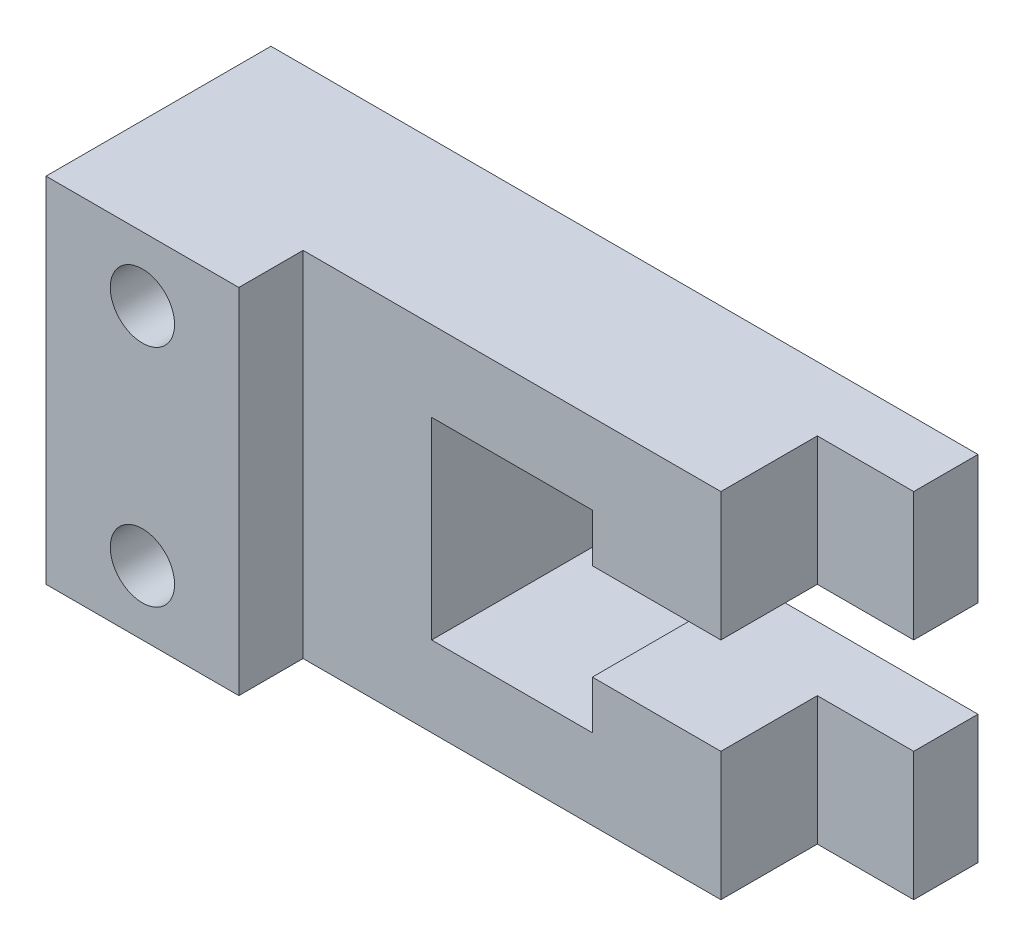
ISO-10303-21;
HEADER;
FILE_DESCRIPTION(('STEP AP214'),'2;1');
FILE_NAME('part.step','',(''),(''),'','','');
FILE_SCHEMA(('AUTOMOTIVE_DESIGN { 1 0 10303 214 1 1 1 1 }'));
ENDSEC;
DATA;
#1=APPLICATION_CONTEXT('core data for automotive mechanical design processes');
#2=APPLICATION_PROTOCOL_DEFINITION('international standard','automotive_design',2000,#1);
#3=PRODUCT_CONTEXT('',#1,'mechanical');
#4=PRODUCT('Part','Part','',(#3));
#5=PRODUCT_RELATED_PRODUCT_CATEGORY('part','',(#4));
#6=PRODUCT_DEFINITION_FORMATION('','',#4);
#7=PRODUCT_DEFINITION_CONTEXT('part definition',#1,'design');
#8=PRODUCT_DEFINITION('design','',#6,#7);
#9=PRODUCT_DEFINITION_SHAPE('','',#8);
#10=(LENGTH_UNIT() NAMED_UNIT(*) SI_UNIT(.MILLI.,.METRE.));
#11=(NAMED_UNIT(*) PLANE_ANGLE_UNIT() SI_UNIT($,.RADIAN.));
#12=(NAMED_UNIT(*) SI_UNIT($,.STERADIAN.) SOLID_ANGLE_UNIT());
#13=UNCERTAINTY_MEASURE_WITH_UNIT(LENGTH_MEASURE(1.E-05),#10,'distance_accuracy_value','');
#14=(GEOMETRIC_REPRESENTATION_CONTEXT(3) GLOBAL_UNCERTAINTY_ASSIGNED_CONTEXT((#13)) GLOBAL_UNIT_ASSIGNED_CONTEXT((#10,
#11,#12)) REPRESENTATION_CONTEXT('',''));
#15=CARTESIAN_POINT('',(0.,0.,0.));
#16=DIRECTION('',(0.,0.,1.));
#17=DIRECTION('',(1.,0.,0.));
#18=AXIS2_PLACEMENT_3D('',#15,#16,#17);
#19=CARTESIAN_POINT('',(0.,0.,10.));
#20=DIRECTION('',(0.,0.,1.));
#21=DIRECTION('',(1.,0.,0.));
#22=AXIS2_PLACEMENT_3D('',#19,#20,#21);
#23=PLANE('',#22);
#24=DIRECTION('',(-1.,0.,0.));
#25=VECTOR('',#24,1.);
#26=CARTESIAN_POINT('',(110.,-35.,10.));
#27=LINE('',#26,#25);
#28=CARTESIAN_POINT('',(110.,-35.,10.));
#29=VERTEX_POINT('',#28);
#30=CARTESIAN_POINT('',(95.,-35.,10.));
#31=VERTEX_POINT('',#30);
#32=EDGE_CURVE('E213',#29,#31,#27,.T.);
#33=ORIENTED_EDGE('',*,*,#32,.T.);
#34=DIRECTION('',(0.,1.,0.));
#35=VECTOR('',#34,1.);
#36=CARTESIAN_POINT('',(95.,-55.,10.));
#37=LINE('',#36,#35);
#38=CARTESIAN_POINT('',(95.,-55.,10.));
#39=VERTEX_POINT('',#38);
#40=EDGE_CURVE('E293',#39,#31,#37,.T.);
#41=ORIENTED_EDGE('',*,*,#40,.F.);
#42=DIRECTION('',(1.,0.,0.));
#43=VECTOR('',#42,1.);
#44=CARTESIAN_POINT('',(0.,-55.,10.));
#45=LINE('',#44,#43);
#46=CARTESIAN_POINT('',(110.,-55.,10.));
#47=VERTEX_POINT('',#46);
#48=EDGE_CURVE('E125',#39,#47,#45,.T.);
#49=ORIENTED_EDGE('',*,*,#48,.T.);
#50=DIRECTION('',(0.,1.,0.));
#51=VECTOR('',#50,1.);
#52=CARTESIAN_POINT('',(110.,-55.,10.));
#53=LINE('',#52,#51);
#54=EDGE_CURVE('E214',#47,#29,#53,.T.);
#55=ORIENTED_EDGE('',*,*,#54,.T.);
#56=EDGE_LOOP('',(#33,#41,#49,#55));
#57=FACE_BOUND('',#56,.T.);
#58=ADVANCED_FACE('F44',(#57),#23,.T.);
#59=DIRECTION('',(-1.,0.,0.));
#60=VECTOR('',#59,1.);
#61=CARTESIAN_POINT('',(110.,0.,10.));
#62=LINE('',#61,#60);
#63=CARTESIAN_POINT('',(110.,0.,10.));
#64=VERTEX_POINT('',#63);
#65=CARTESIAN_POINT('',(95.,0.,10.));
#66=VERTEX_POINT('',#65);
#67=EDGE_CURVE('E208',#64,#66,#62,.T.);
#68=ORIENTED_EDGE('',*,*,#67,.T.);
#69=DIRECTION('',(0.,1.,0.));
#70=VECTOR('',#69,1.);
#71=CARTESIAN_POINT('',(95.,-20.,10.));
#72=LINE('',#71,#70);
#73=CARTESIAN_POINT('',(95.,-20.,10.));
#74=VERTEX_POINT('',#73);
#75=EDGE_CURVE('E291',#74,#66,#72,.T.);
#76=ORIENTED_EDGE('',*,*,#75,.F.);
#77=DIRECTION('',(1.,0.,0.));
#78=VECTOR('',#77,1.);
#79=CARTESIAN_POINT('',(75.,-20.,10.));
#80=LINE('',#79,#78);
#81=CARTESIAN_POINT('',(110.,-20.,10.));
#82=VERTEX_POINT('',#81);
#83=EDGE_CURVE('E217',#74,#82,#80,.T.);
#84=ORIENTED_EDGE('',*,*,#83,.T.);
#85=DIRECTION('',(0.,1.,0.));
#86=VECTOR('',#85,1.);
#87=CARTESIAN_POINT('',(110.,-20.,10.));
#88=LINE('',#87,#86);
#89=EDGE_CURVE('E68',#82,#64,#88,.T.);
#90=ORIENTED_EDGE('',*,*,#89,.T.);
#91=EDGE_LOOP('',(#68,#76,#84,#90));
#92=FACE_BOUND('',#91,.T.);
#93=ADVANCED_FACE('F335',(#92),#23,.T.);
#94=CARTESIAN_POINT('',(110.,0.,10.));
#95=DIRECTION('',(0.,-1.,0.));
#96=DIRECTION('',(0.,0.,-1.));
#97=AXIS2_PLACEMENT_3D('',#94,#95,#96);
#98=PLANE('',#97);
#99=DIRECTION('',(-1.,0.,0.));
#100=VECTOR('',#99,1.);
#101=CARTESIAN_POINT('',(110.,0.,0.));
#102=LINE('',#101,#100);
#103=CARTESIAN_POINT('',(110.,0.,0.));
#104=VERTEX_POINT('',#103);
#105=CARTESIAN_POINT('',(0.,0.,0.));
#106=VERTEX_POINT('',#105);
#107=EDGE_CURVE('E199',#104,#106,#102,.T.);
#108=ORIENTED_EDGE('',*,*,#107,.T.);
#109=DIRECTION('',(0.,0.,-1.));
#110=VECTOR('',#109,1.);
#111=CARTESIAN_POINT('',(0.,0.,10.));
#112=LINE('',#111,#110);
#113=CARTESIAN_POINT('',(0.,0.,35.));
#114=VERTEX_POINT('',#113);
#115=EDGE_CURVE('E11',#114,#106,#112,.T.);
#116=ORIENTED_EDGE('',*,*,#115,.F.);
#117=DIRECTION('',(-1.,0.,0.));
#118=VECTOR('',#117,1.);
#119=CARTESIAN_POINT('',(0.,0.,35.));
#120=LINE('',#119,#118);
#121=CARTESIAN_POINT('',(30.,0.,35.));
#122=VERTEX_POINT('',#121);
#123=EDGE_CURVE('E207',#122,#114,#120,.T.);
#124=ORIENTED_EDGE('',*,*,#123,.F.);
#125=DIRECTION('',(0.,0.,-1.));
#126=VECTOR('',#125,1.);
#127=CARTESIAN_POINT('',(30.,0.,35.));
#128=LINE('',#127,#126);
#129=CARTESIAN_POINT('',(30.,0.,25.));
#130=VERTEX_POINT('',#129);
#131=EDGE_CURVE('E202',#122,#130,#128,.T.);
#132=ORIENTED_EDGE('',*,*,#131,.T.);
#133=DIRECTION('',(-1.,0.,0.));
#134=VECTOR('',#133,1.);
#135=CARTESIAN_POINT('',(95.,0.,25.));
#136=LINE('',#135,#134);
#137=CARTESIAN_POINT('',(95.,0.,25.));
#138=VERTEX_POINT('',#137);
#139=EDGE_CURVE('E58',#138,#130,#136,.T.);
#140=ORIENTED_EDGE('',*,*,#139,.F.);
#141=DIRECTION('',(0.,0.,-1.));
#142=VECTOR('',#141,1.);
#143=CARTESIAN_POINT('',(95.,0.,25.));
#144=LINE('',#143,#142);
#145=EDGE_CURVE('E302',#138,#66,#144,.T.);
#146=ORIENTED_EDGE('',*,*,#145,.T.);
#147=ORIENTED_EDGE('',*,*,#67,.F.);
#148=DIRECTION('',(0.,0.,-1.));
#149=VECTOR('',#148,1.);
#150=CARTESIAN_POINT('',(110.,0.,10.));
#151=LINE('',#150,#149);
#152=EDGE_CURVE('E219',#64,#104,#151,.T.);
#153=ORIENTED_EDGE('',*,*,#152,.T.);
#154=EDGE_LOOP('',(#108,#116,#124,#132,#140,#146,#147,#153));
#155=FACE_BOUND('',#154,.T.);
#156=ADVANCED_FACE('F50',(#155),#98,.F.);
#157=CARTESIAN_POINT('',(0.,0.,10.));
#158=DIRECTION('',(1.,0.,0.));
#159=DIRECTION('',(0.,0.,-1.));
#160=AXIS2_PLACEMENT_3D('',#157,#158,#159);
#161=PLANE('',#160);
#162=DIRECTION('',(0.,-1.,0.));
#163=VECTOR('',#162,1.);
#164=CARTESIAN_POINT('',(0.,0.,0.));
#165=LINE('',#164,#163);
#166=CARTESIAN_POINT('',(0.,-55.,0.));
#167=VERTEX_POINT('',#166);
#168=EDGE_CURVE('E201',#106,#167,#165,.T.);
#169=ORIENTED_EDGE('',*,*,#168,.T.);
#170=DIRECTION('',(0.,0.,-1.));
#171=VECTOR('',#170,1.);
#172=CARTESIAN_POINT('',(0.,-55.,10.));
#173=LINE('',#172,#171);
#174=CARTESIAN_POINT('',(0.,-55.,35.));
#175=VERTEX_POINT('',#174);
#176=EDGE_CURVE('E52',#175,#167,#173,.T.);
#177=ORIENTED_EDGE('',*,*,#176,.F.);
#178=DIRECTION('',(0.,-1.,0.));
#179=VECTOR('',#178,1.);
#180=CARTESIAN_POINT('',(0.,0.,35.));
#181=LINE('',#180,#179);
#182=EDGE_CURVE('E311',#114,#175,#181,.T.);
#183=ORIENTED_EDGE('',*,*,#182,.F.);
#184=ORIENTED_EDGE('',*,*,#115,.T.);
#185=EDGE_LOOP('',(#169,#177,#183,#184));
#186=FACE_BOUND('',#185,.T.);
#187=ADVANCED_FACE('F316',(#186),#161,.F.);
#188=CARTESIAN_POINT('',(0.,-55.,10.));
#189=DIRECTION('',(0.,1.,0.));
#190=DIRECTION('',(0.,0.,1.));
#191=AXIS2_PLACEMENT_3D('',#188,#189,#190);
#192=PLANE('',#191);
#193=ORIENTED_EDGE('',*,*,#48,.F.);
#194=DIRECTION('',(0.,0.,-1.));
#195=VECTOR('',#194,1.);
#196=CARTESIAN_POINT('',(95.,-55.,25.));
#197=LINE('',#196,#195);
#198=CARTESIAN_POINT('',(95.,-55.,25.));
#199=VERTEX_POINT('',#198);
#200=EDGE_CURVE('E191',#199,#39,#197,.T.);
#201=ORIENTED_EDGE('',*,*,#200,.F.);
#202=DIRECTION('',(1.,0.,0.));
#203=VECTOR('',#202,1.);
#204=CARTESIAN_POINT('',(30.,-55.,25.));
#205=LINE('',#204,#203);
#206=CARTESIAN_POINT('',(30.,-55.,25.));
#207=VERTEX_POINT('',#206);
#208=EDGE_CURVE('E181',#207,#199,#205,.T.);
#209=ORIENTED_EDGE('',*,*,#208,.F.);
#210=DIRECTION('',(0.,0.,-1.));
#211=VECTOR('',#210,1.);
#212=CARTESIAN_POINT('',(30.,-55.,35.));
#213=LINE('',#212,#211);
#214=CARTESIAN_POINT('',(30.,-55.,35.));
#215=VERTEX_POINT('',#214);
#216=EDGE_CURVE('E195',#215,#207,#213,.T.);
#217=ORIENTED_EDGE('',*,*,#216,.F.);
#218=DIRECTION('',(1.,0.,0.));
#219=VECTOR('',#218,1.);
#220=CARTESIAN_POINT('',(0.,-55.,35.));
#221=LINE('',#220,#219);
#222=EDGE_CURVE('E268',#175,#215,#221,.T.);
#223=ORIENTED_EDGE('',*,*,#222,.F.);
#224=ORIENTED_EDGE('',*,*,#176,.T.);
#225=DIRECTION('',(1.,0.,0.));
#226=VECTOR('',#225,1.);
#227=CARTESIAN_POINT('',(0.,-55.,0.));
#228=LINE('',#227,#226);
#229=CARTESIAN_POINT('',(110.,-55.,0.));
#230=VERTEX_POINT('',#229);
#231=EDGE_CURVE('E224',#167,#230,#228,.T.);
#232=ORIENTED_EDGE('',*,*,#231,.T.);
#233=DIRECTION('',(0.,0.,-1.));
#234=VECTOR('',#233,1.);
#235=CARTESIAN_POINT('',(110.,-55.,10.));
#236=LINE('',#235,#234);
#237=EDGE_CURVE('E267',#47,#230,#236,.T.);
#238=ORIENTED_EDGE('',*,*,#237,.F.);
#239=EDGE_LOOP('',(#193,#201,#209,#217,#223,#224,#232,#238));
#240=FACE_BOUND('',#239,.T.);
#241=ADVANCED_FACE('F188',(#240),#192,.F.);
#242=CARTESIAN_POINT('',(110.,-55.,10.));
#243=DIRECTION('',(-1.,0.,0.));
#244=DIRECTION('',(0.,0.,1.));
#245=AXIS2_PLACEMENT_3D('',#242,#243,#244);
#246=PLANE('',#245);
#247=DIRECTION('',(0.,1.,0.));
#248=VECTOR('',#247,1.);
#249=CARTESIAN_POINT('',(110.,-55.,0.));
#250=LINE('',#249,#248);
#251=CARTESIAN_POINT('',(110.,-35.,0.));
#252=VERTEX_POINT('',#251);
#253=EDGE_CURVE('E223',#230,#252,#250,.T.);
#254=ORIENTED_EDGE('',*,*,#253,.T.);
#255=DIRECTION('',(0.,0.,-1.));
#256=VECTOR('',#255,1.);
#257=CARTESIAN_POINT('',(110.,-35.,10.));
#258=LINE('',#257,#256);
#259=EDGE_CURVE('E262',#29,#252,#258,.T.);
#260=ORIENTED_EDGE('',*,*,#259,.F.);
#261=ORIENTED_EDGE('',*,*,#54,.F.);
#262=ORIENTED_EDGE('',*,*,#237,.T.);
#263=EDGE_LOOP('',(#254,#260,#261,#262));
#264=FACE_BOUND('',#263,.T.);
#265=ADVANCED_FACE('F285',(#264),#246,.F.);
#266=CARTESIAN_POINT('',(110.,-35.,10.));
#267=DIRECTION('',(0.,-1.,0.));
#268=DIRECTION('',(0.,0.,-1.));
#269=AXIS2_PLACEMENT_3D('',#266,#267,#268);
#270=PLANE('',#269);
#271=DIRECTION('',(-1.,0.,0.));
#272=VECTOR('',#271,1.);
#273=CARTESIAN_POINT('',(110.,-35.,0.));
#274=LINE('',#273,#272);
#275=CARTESIAN_POINT('',(75.,-35.,0.));
#276=VERTEX_POINT('',#275);
#277=EDGE_CURVE('E227',#252,#276,#274,.T.);
#278=ORIENTED_EDGE('',*,*,#277,.T.);
#279=DIRECTION('',(0.,0.,-1.));
#280=VECTOR('',#279,1.);
#281=CARTESIAN_POINT('',(75.,-35.,10.));
#282=LINE('',#281,#280);
#283=CARTESIAN_POINT('',(75.,-35.,25.));
#284=VERTEX_POINT('',#283);
#285=EDGE_CURVE('E258',#284,#276,#282,.T.);
#286=ORIENTED_EDGE('',*,*,#285,.F.);
#287=DIRECTION('',(-1.,0.,0.));
#288=VECTOR('',#287,1.);
#289=CARTESIAN_POINT('',(95.,-35.,25.));
#290=LINE('',#289,#288);
#291=CARTESIAN_POINT('',(95.,-35.,25.));
#292=VERTEX_POINT('',#291);
#293=EDGE_CURVE('E351',#292,#284,#290,.T.);
#294=ORIENTED_EDGE('',*,*,#293,.F.);
#295=DIRECTION('',(0.,0.,-1.));
#296=VECTOR('',#295,1.);
#297=CARTESIAN_POINT('',(95.,-35.,25.));
#298=LINE('',#297,#296);
#299=EDGE_CURVE('E288',#292,#31,#298,.T.);
#300=ORIENTED_EDGE('',*,*,#299,.T.);
#301=ORIENTED_EDGE('',*,*,#32,.F.);
#302=ORIENTED_EDGE('',*,*,#259,.T.);
#303=EDGE_LOOP('',(#278,#286,#294,#300,#301,#302));
#304=FACE_BOUND('',#303,.T.);
#305=ADVANCED_FACE('F287',(#304),#270,.F.);
#306=CARTESIAN_POINT('',(75.,-35.,10.));
#307=DIRECTION('',(1.,0.,0.));
#308=DIRECTION('',(0.,0.,-1.));
#309=AXIS2_PLACEMENT_3D('',#306,#307,#308);
#310=PLANE('',#309);
#311=DIRECTION('',(0.,-1.,0.));
#312=VECTOR('',#311,1.);
#313=CARTESIAN_POINT('',(75.,-35.,0.));
#314=LINE('',#313,#312);
#315=CARTESIAN_POINT('',(75.,-42.5,0.));
#316=VERTEX_POINT('',#315);
#317=EDGE_CURVE('E230',#276,#316,#314,.T.);
#318=ORIENTED_EDGE('',*,*,#317,.T.);
#319=DIRECTION('',(0.,0.,-1.));
#320=VECTOR('',#319,1.);
#321=CARTESIAN_POINT('',(75.,-42.5,10.));
#322=LINE('',#321,#320);
#323=CARTESIAN_POINT('',(75.,-42.5,25.));
#324=VERTEX_POINT('',#323);
#325=EDGE_CURVE('E260',#324,#316,#322,.T.);
#326=ORIENTED_EDGE('',*,*,#325,.F.);
#327=DIRECTION('',(0.,-1.,0.));
#328=VECTOR('',#327,1.);
#329=CARTESIAN_POINT('',(75.,-35.,25.));
#330=LINE('',#329,#328);
#331=EDGE_CURVE('E352',#284,#324,#330,.T.);
#332=ORIENTED_EDGE('',*,*,#331,.F.);
#333=ORIENTED_EDGE('',*,*,#285,.T.);
#334=EDGE_LOOP('',(#318,#326,#332,#333));
#335=FACE_BOUND('',#334,.T.);
#336=ADVANCED_FACE('F494',(#335),#310,.F.);
#337=CARTESIAN_POINT('',(75.,-42.5,10.));
#338=DIRECTION('',(0.,-1.,0.));
#339=DIRECTION('',(0.,0.,-1.));
#340=AXIS2_PLACEMENT_3D('',#337,#338,#339);
#341=PLANE('',#340);
#342=DIRECTION('',(-1.,0.,0.));
#343=VECTOR('',#342,1.);
#344=CARTESIAN_POINT('',(75.,-42.5,0.));
#345=LINE('',#344,#343);
#346=CARTESIAN_POINT('',(50.,-42.5,0.));
#347=VERTEX_POINT('',#346);
#348=EDGE_CURVE('E233',#316,#347,#345,.T.);
#349=ORIENTED_EDGE('',*,*,#348,.T.);
#350=DIRECTION('',(0.,0.,-1.));
#351=VECTOR('',#350,1.);
#352=CARTESIAN_POINT('',(50.,-42.5,10.));
#353=LINE('',#352,#351);
#354=CARTESIAN_POINT('',(50.,-42.5,25.));
#355=VERTEX_POINT('',#354);
#356=EDGE_CURVE('E251',#355,#347,#353,.T.);
#357=ORIENTED_EDGE('',*,*,#356,.F.);
#358=DIRECTION('',(-1.,0.,0.));
#359=VECTOR('',#358,1.);
#360=CARTESIAN_POINT('',(75.,-42.5,25.));
#361=LINE('',#360,#359);
#362=EDGE_CURVE('E347',#324,#355,#361,.T.);
#363=ORIENTED_EDGE('',*,*,#362,.F.);
#364=ORIENTED_EDGE('',*,*,#325,.T.);
#365=EDGE_LOOP('',(#349,#357,#363,#364));
#366=FACE_BOUND('',#365,.T.);
#367=ADVANCED_FACE('F481',(#366),#341,.F.);
#368=CARTESIAN_POINT('',(50.,-42.5,10.));
#369=DIRECTION('',(-1.,0.,0.));
#370=DIRECTION('',(0.,0.,1.));
#371=AXIS2_PLACEMENT_3D('',#368,#369,#370);
#372=PLANE('',#371);
#373=DIRECTION('',(0.,1.,0.));
#374=VECTOR('',#373,1.);
#375=CARTESIAN_POINT('',(50.,-42.5,0.));
#376=LINE('',#375,#374);
#377=CARTESIAN_POINT('',(50.,-12.5,0.));
#378=VERTEX_POINT('',#377);
#379=EDGE_CURVE('E231',#347,#378,#376,.T.);
#380=ORIENTED_EDGE('',*,*,#379,.T.);
#381=DIRECTION('',(0.,0.,-1.));
#382=VECTOR('',#381,1.);
#383=CARTESIAN_POINT('',(50.,-12.5,10.));
#384=LINE('',#383,#382);
#385=CARTESIAN_POINT('',(50.,-12.5,25.));
#386=VERTEX_POINT('',#385);
#387=EDGE_CURVE('E252',#386,#378,#384,.T.);
#388=ORIENTED_EDGE('',*,*,#387,.F.);
#389=DIRECTION('',(0.,1.,0.));
#390=VECTOR('',#389,1.);
#391=CARTESIAN_POINT('',(50.,-42.5,25.));
#392=LINE('',#391,#390);
#393=EDGE_CURVE('E343',#355,#386,#392,.T.);
#394=ORIENTED_EDGE('',*,*,#393,.F.);
#395=ORIENTED_EDGE('',*,*,#356,.T.);
#396=EDGE_LOOP('',(#380,#388,#394,#395));
#397=FACE_BOUND('',#396,.T.);
#398=ADVANCED_FACE('F474',(#397),#372,.F.);
#399=CARTESIAN_POINT('',(50.,-12.5,10.));
#400=DIRECTION('',(0.,1.,0.));
#401=DIRECTION('',(0.,0.,1.));
#402=AXIS2_PLACEMENT_3D('',#399,#400,#401);
#403=PLANE('',#402);
#404=DIRECTION('',(1.,0.,0.));
#405=VECTOR('',#404,1.);
#406=CARTESIAN_POINT('',(50.,-12.5,0.));
#407=LINE('',#406,#405);
#408=CARTESIAN_POINT('',(75.,-12.5,0.));
#409=VERTEX_POINT('',#408);
#410=EDGE_CURVE('E232',#378,#409,#407,.T.);
#411=ORIENTED_EDGE('',*,*,#410,.T.);
#412=DIRECTION('',(0.,0.,-1.));
#413=VECTOR('',#412,1.);
#414=CARTESIAN_POINT('',(75.,-12.5,10.));
#415=LINE('',#414,#413);
#416=CARTESIAN_POINT('',(75.,-12.5,25.));
#417=VERTEX_POINT('',#416);
#418=EDGE_CURVE('E247',#417,#409,#415,.T.);
#419=ORIENTED_EDGE('',*,*,#418,.F.);
#420=DIRECTION('',(1.,0.,0.));
#421=VECTOR('',#420,1.);
#422=CARTESIAN_POINT('',(50.,-12.5,25.));
#423=LINE('',#422,#421);
#424=EDGE_CURVE('E338',#386,#417,#423,.T.);
#425=ORIENTED_EDGE('',*,*,#424,.F.);
#426=ORIENTED_EDGE('',*,*,#387,.T.);
#427=EDGE_LOOP('',(#411,#419,#425,#426));
#428=FACE_BOUND('',#427,.T.);
#429=ADVANCED_FACE('F464',(#428),#403,.F.);
#430=CARTESIAN_POINT('',(75.,-12.5,10.));
#431=DIRECTION('',(1.,0.,0.));
#432=DIRECTION('',(0.,0.,-1.));
#433=AXIS2_PLACEMENT_3D('',#430,#431,#432);
#434=PLANE('',#433);
#435=DIRECTION('',(0.,-1.,0.));
#436=VECTOR('',#435,1.);
#437=CARTESIAN_POINT('',(75.,-12.5,0.));
#438=LINE('',#437,#436);
#439=CARTESIAN_POINT('',(75.,-20.,0.));
#440=VERTEX_POINT('',#439);
#441=EDGE_CURVE('E240',#409,#440,#438,.T.);
#442=ORIENTED_EDGE('',*,*,#441,.T.);
#443=DIRECTION('',(0.,0.,-1.));
#444=VECTOR('',#443,1.);
#445=CARTESIAN_POINT('',(75.,-20.,10.));
#446=LINE('',#445,#444);
#447=CARTESIAN_POINT('',(75.,-20.,25.));
#448=VERTEX_POINT('',#447);
#449=EDGE_CURVE('E244',#448,#440,#446,.T.);
#450=ORIENTED_EDGE('',*,*,#449,.F.);
#451=DIRECTION('',(0.,-1.,0.));
#452=VECTOR('',#451,1.);
#453=CARTESIAN_POINT('',(75.,-12.5,25.));
#454=LINE('',#453,#452);
#455=EDGE_CURVE('E336',#417,#448,#454,.T.);
#456=ORIENTED_EDGE('',*,*,#455,.F.);
#457=ORIENTED_EDGE('',*,*,#418,.T.);
#458=EDGE_LOOP('',(#442,#450,#456,#457));
#459=FACE_BOUND('',#458,.T.);
#460=ADVANCED_FACE('F451',(#459),#434,.F.);
#461=CARTESIAN_POINT('',(75.,-20.,10.));
#462=DIRECTION('',(0.,1.,0.));
#463=DIRECTION('',(0.,0.,1.));
#464=AXIS2_PLACEMENT_3D('',#461,#462,#463);
#465=PLANE('',#464);
#466=DIRECTION('',(1.,0.,0.));
#467=VECTOR('',#466,1.);
#468=CARTESIAN_POINT('',(75.,-20.,0.));
#469=LINE('',#468,#467);
#470=CARTESIAN_POINT('',(110.,-20.,0.));
#471=VERTEX_POINT('',#470);
#472=EDGE_CURVE('E237',#440,#471,#469,.T.);
#473=ORIENTED_EDGE('',*,*,#472,.T.);
#474=DIRECTION('',(0.,0.,-1.));
#475=VECTOR('',#474,1.);
#476=CARTESIAN_POINT('',(110.,-20.,10.));
#477=LINE('',#476,#475);
#478=EDGE_CURVE('E243',#82,#471,#477,.T.);
#479=ORIENTED_EDGE('',*,*,#478,.F.);
#480=ORIENTED_EDGE('',*,*,#83,.F.);
#481=DIRECTION('',(0.,0.,-1.));
#482=VECTOR('',#481,1.);
#483=CARTESIAN_POINT('',(95.,-20.,25.));
#484=LINE('',#483,#482);
#485=CARTESIAN_POINT('',(95.,-20.,25.));
#486=VERTEX_POINT('',#485);
#487=EDGE_CURVE('E310',#486,#74,#484,.T.);
#488=ORIENTED_EDGE('',*,*,#487,.F.);
#489=DIRECTION('',(1.,0.,0.));
#490=VECTOR('',#489,1.);
#491=CARTESIAN_POINT('',(75.,-20.,25.));
#492=LINE('',#491,#490);
#493=EDGE_CURVE('E337',#448,#486,#492,.T.);
#494=ORIENTED_EDGE('',*,*,#493,.F.);
#495=ORIENTED_EDGE('',*,*,#449,.T.);
#496=EDGE_LOOP('',(#473,#479,#480,#488,#494,#495));
#497=FACE_BOUND('',#496,.T.);
#498=ADVANCED_FACE('F326',(#497),#465,.F.);
#499=CARTESIAN_POINT('',(110.,-20.,10.));
#500=DIRECTION('',(-1.,0.,0.));
#501=DIRECTION('',(0.,0.,1.));
#502=AXIS2_PLACEMENT_3D('',#499,#500,#501);
#503=PLANE('',#502);
#504=DIRECTION('',(0.,1.,0.));
#505=VECTOR('',#504,1.);
#506=CARTESIAN_POINT('',(110.,-20.,0.));
#507=LINE('',#506,#505);
#508=EDGE_CURVE('E112',#471,#104,#507,.T.);
#509=ORIENTED_EDGE('',*,*,#508,.T.);
#510=ORIENTED_EDGE('',*,*,#152,.F.);
#511=ORIENTED_EDGE('',*,*,#89,.F.);
#512=ORIENTED_EDGE('',*,*,#478,.T.);
#513=EDGE_LOOP('',(#509,#510,#511,#512));
#514=FACE_BOUND('',#513,.T.);
#515=ADVANCED_FACE('F328',(#514),#503,.F.);
#516=CARTESIAN_POINT('',(0.,0.,0.));
#517=DIRECTION('',(0.,0.,1.));
#518=DIRECTION('',(1.,0.,0.));
#519=AXIS2_PLACEMENT_3D('',#516,#517,#518);
#520=PLANE('',#519);
#521=CARTESIAN_POINT('',(15.,-10.,0.));
#522=DIRECTION('',(0.,0.,1.));
#523=DIRECTION('',(1.,0.,0.));
#524=AXIS2_PLACEMENT_3D('',#521,#522,#523);
#525=CIRCLE('',#524,5.);
#526=CARTESIAN_POINT('',(20.,-10.,0.));
#527=VERTEX_POINT('',#526);
#528=EDGE_CURVE('E295',#527,#527,#525,.T.);
#529=ORIENTED_EDGE('',*,*,#528,.T.);
#530=EDGE_LOOP('',(#529));
#531=FACE_BOUND('',#530,.T.);
#532=CARTESIAN_POINT('',(15.,-45.,0.));
#533=DIRECTION('',(0.,0.,1.));
#534=DIRECTION('',(1.,0.,0.));
#535=AXIS2_PLACEMENT_3D('',#532,#533,#534);
#536=CIRCLE('',#535,5.00000000000001);
#537=CARTESIAN_POINT('',(20.,-45.,0.));
#538=VERTEX_POINT('',#537);
#539=EDGE_CURVE('E296',#538,#538,#536,.T.);
#540=ORIENTED_EDGE('',*,*,#539,.T.);
#541=EDGE_LOOP('',(#540));
#542=FACE_BOUND('',#541,.T.);
#543=ORIENTED_EDGE('',*,*,#107,.F.);
#544=ORIENTED_EDGE('',*,*,#508,.F.);
#545=ORIENTED_EDGE('',*,*,#472,.F.);
#546=ORIENTED_EDGE('',*,*,#441,.F.);
#547=ORIENTED_EDGE('',*,*,#410,.F.);
#548=ORIENTED_EDGE('',*,*,#379,.F.);
#549=ORIENTED_EDGE('',*,*,#348,.F.);
#550=ORIENTED_EDGE('',*,*,#317,.F.);
#551=ORIENTED_EDGE('',*,*,#277,.F.);
#552=ORIENTED_EDGE('',*,*,#253,.F.);
#553=ORIENTED_EDGE('',*,*,#231,.F.);
#554=ORIENTED_EDGE('',*,*,#168,.F.);
#555=EDGE_LOOP('',(#543,#544,#545,#546,#547,#548,#549,#550,#551,#552,#553,#554));
#556=FACE_BOUND('',#555,.T.);
#557=ADVANCED_FACE('F280',(#531,#542,#556),#520,.F.);
#558=CARTESIAN_POINT('',(30.,0.,35.));
#559=DIRECTION('',(-1.,0.,0.));
#560=DIRECTION('',(0.,-1.,0.));
#561=AXIS2_PLACEMENT_3D('',#558,#559,#560);
#562=PLANE('',#561);
#563=ORIENTED_EDGE('',*,*,#216,.T.);
#564=DIRECTION('',(0.,-1.,0.));
#565=VECTOR('',#564,1.);
#566=CARTESIAN_POINT('',(30.,0.,25.));
#567=LINE('',#566,#565);
#568=EDGE_CURVE('E178',#130,#207,#567,.T.);
#569=ORIENTED_EDGE('',*,*,#568,.F.);
#570=ORIENTED_EDGE('',*,*,#131,.F.);
#571=DIRECTION('',(0.,1.,0.));
#572=VECTOR('',#571,1.);
#573=CARTESIAN_POINT('',(30.,0.,35.));
#574=LINE('',#573,#572);
#575=EDGE_CURVE('E198',#215,#122,#574,.T.);
#576=ORIENTED_EDGE('',*,*,#575,.F.);
#577=EDGE_LOOP('',(#563,#569,#570,#576));
#578=FACE_BOUND('',#577,.T.);
#579=ADVANCED_FACE('F197',(#578),#562,.F.);
#580=CARTESIAN_POINT('',(0.,0.,35.));
#581=DIRECTION('',(0.,0.,1.));
#582=DIRECTION('',(1.,0.,0.));
#583=AXIS2_PLACEMENT_3D('',#580,#581,#582);
#584=PLANE('',#583);
#585=CARTESIAN_POINT('',(15.,-10.,35.));
#586=DIRECTION('',(0.,0.,1.));
#587=DIRECTION('',(1.,0.,0.));
#588=AXIS2_PLACEMENT_3D('',#585,#586,#587);
#589=CIRCLE('',#588,5.);
#590=CARTESIAN_POINT('',(20.,-10.,35.));
#591=VERTEX_POINT('',#590);
#592=EDGE_CURVE('E363',#591,#591,#589,.T.);
#593=ORIENTED_EDGE('',*,*,#592,.F.);
#594=EDGE_LOOP('',(#593));
#595=FACE_BOUND('',#594,.T.);
#596=CARTESIAN_POINT('',(15.,-45.,35.));
#597=DIRECTION('',(0.,0.,1.));
#598=DIRECTION('',(1.,0.,0.));
#599=AXIS2_PLACEMENT_3D('',#596,#597,#598);
#600=CIRCLE('',#599,5.00000000000001);
#601=CARTESIAN_POINT('',(20.,-45.,35.));
#602=VERTEX_POINT('',#601);
#603=EDGE_CURVE('E365',#602,#602,#600,.T.);
#604=ORIENTED_EDGE('',*,*,#603,.F.);
#605=EDGE_LOOP('',(#604));
#606=FACE_BOUND('',#605,.T.);
#607=ORIENTED_EDGE('',*,*,#182,.T.);
#608=ORIENTED_EDGE('',*,*,#222,.T.);
#609=ORIENTED_EDGE('',*,*,#575,.T.);
#610=ORIENTED_EDGE('',*,*,#123,.T.);
#611=EDGE_LOOP('',(#607,#608,#609,#610));
#612=FACE_BOUND('',#611,.T.);
#613=ADVANCED_FACE('F320',(#595,#606,#612),#584,.T.);
#614=CARTESIAN_POINT('',(95.,-55.,25.));
#615=DIRECTION('',(-1.,0.,0.));
#616=DIRECTION('',(0.,0.,1.));
#617=AXIS2_PLACEMENT_3D('',#614,#615,#616);
#618=PLANE('',#617);
#619=ORIENTED_EDGE('',*,*,#40,.T.);
#620=ORIENTED_EDGE('',*,*,#299,.F.);
#621=DIRECTION('',(0.,1.,0.));
#622=VECTOR('',#621,1.);
#623=CARTESIAN_POINT('',(95.,-55.,25.));
#624=LINE('',#623,#622);
#625=EDGE_CURVE('E196',#199,#292,#624,.T.);
#626=ORIENTED_EDGE('',*,*,#625,.F.);
#627=ORIENTED_EDGE('',*,*,#200,.T.);
#628=EDGE_LOOP('',(#619,#620,#626,#627));
#629=FACE_BOUND('',#628,.T.);
#630=ADVANCED_FACE('F373',(#629),#618,.F.);
#631=CARTESIAN_POINT('',(95.,-20.,25.));
#632=DIRECTION('',(-1.,0.,0.));
#633=DIRECTION('',(0.,0.,1.));
#634=AXIS2_PLACEMENT_3D('',#631,#632,#633);
#635=PLANE('',#634);
#636=ORIENTED_EDGE('',*,*,#75,.T.);
#637=ORIENTED_EDGE('',*,*,#145,.F.);
#638=DIRECTION('',(0.,1.,0.));
#639=VECTOR('',#638,1.);
#640=CARTESIAN_POINT('',(95.,-20.,25.));
#641=LINE('',#640,#639);
#642=EDGE_CURVE('E301',#486,#138,#641,.T.);
#643=ORIENTED_EDGE('',*,*,#642,.F.);
#644=ORIENTED_EDGE('',*,*,#487,.T.);
#645=EDGE_LOOP('',(#636,#637,#643,#644));
#646=FACE_BOUND('',#645,.T.);
#647=ADVANCED_FACE('F340',(#646),#635,.F.);
#648=CARTESIAN_POINT('',(0.,0.,25.));
#649=DIRECTION('',(0.,0.,1.));
#650=DIRECTION('',(1.,0.,0.));
#651=AXIS2_PLACEMENT_3D('',#648,#649,#650);
#652=PLANE('',#651);
#653=ORIENTED_EDGE('',*,*,#139,.T.);
#654=ORIENTED_EDGE('',*,*,#568,.T.);
#655=ORIENTED_EDGE('',*,*,#208,.T.);
#656=ORIENTED_EDGE('',*,*,#625,.T.);
#657=ORIENTED_EDGE('',*,*,#293,.T.);
#658=ORIENTED_EDGE('',*,*,#331,.T.);
#659=ORIENTED_EDGE('',*,*,#362,.T.);
#660=ORIENTED_EDGE('',*,*,#393,.T.);
#661=ORIENTED_EDGE('',*,*,#424,.T.);
#662=ORIENTED_EDGE('',*,*,#455,.T.);
#663=ORIENTED_EDGE('',*,*,#493,.T.);
#664=ORIENTED_EDGE('',*,*,#642,.T.);
#665=EDGE_LOOP('',(#653,#654,#655,#656,#657,#658,#659,#660,#661,#662,#663,#664));
#666=FACE_BOUND('',#665,.T.);
#667=ADVANCED_FACE('F179',(#666),#652,.T.);
#668=CARTESIAN_POINT('',(15.,-45.,-20.));
#669=DIRECTION('',(0.,0.,1.));
#670=DIRECTION('',(1.,0.,0.));
#671=AXIS2_PLACEMENT_3D('',#668,#669,#670);
#672=CYLINDRICAL_SURFACE('',#671,5.00000000000001);
#673=ORIENTED_EDGE('',*,*,#603,.T.);
#674=EDGE_LOOP('',(#673));
#675=FACE_BOUND('',#674,.T.);
#676=ORIENTED_EDGE('',*,*,#539,.F.);
#677=EDGE_LOOP('',(#676));
#678=FACE_BOUND('',#677,.T.);
#679=ADVANCED_FACE('F380',(#675,#678),#672,.F.);
#680=CARTESIAN_POINT('',(15.,-10.,-20.));
#681=DIRECTION('',(0.,0.,1.));
#682=DIRECTION('',(1.,0.,0.));
#683=AXIS2_PLACEMENT_3D('',#680,#681,#682);
#684=CYLINDRICAL_SURFACE('',#683,5.);
#685=ORIENTED_EDGE('',*,*,#592,.T.);
#686=EDGE_LOOP('',(#685));
#687=FACE_BOUND('',#686,.T.);
#688=ORIENTED_EDGE('',*,*,#528,.F.);
#689=EDGE_LOOP('',(#688));
#690=FACE_BOUND('',#689,.T.);
#691=ADVANCED_FACE('F368',(#687,#690),#684,.F.);
#692=CLOSED_SHELL('',(#58,#93,#156,#187,#241,#265,#305,#336,#367,#398,#429,#460,#498,#515,#557,
#579,#613,#630,#647,#667,#679,#691));
#693=MANIFOLD_SOLID_BREP('B2',#692);
#694=ADVANCED_BREP_SHAPE_REPRESENTATION('',(#18,#693),#14);
#695=SHAPE_DEFINITION_REPRESENTATION(#9,#694);
ENDSEC;
END-ISO-10303-21;
